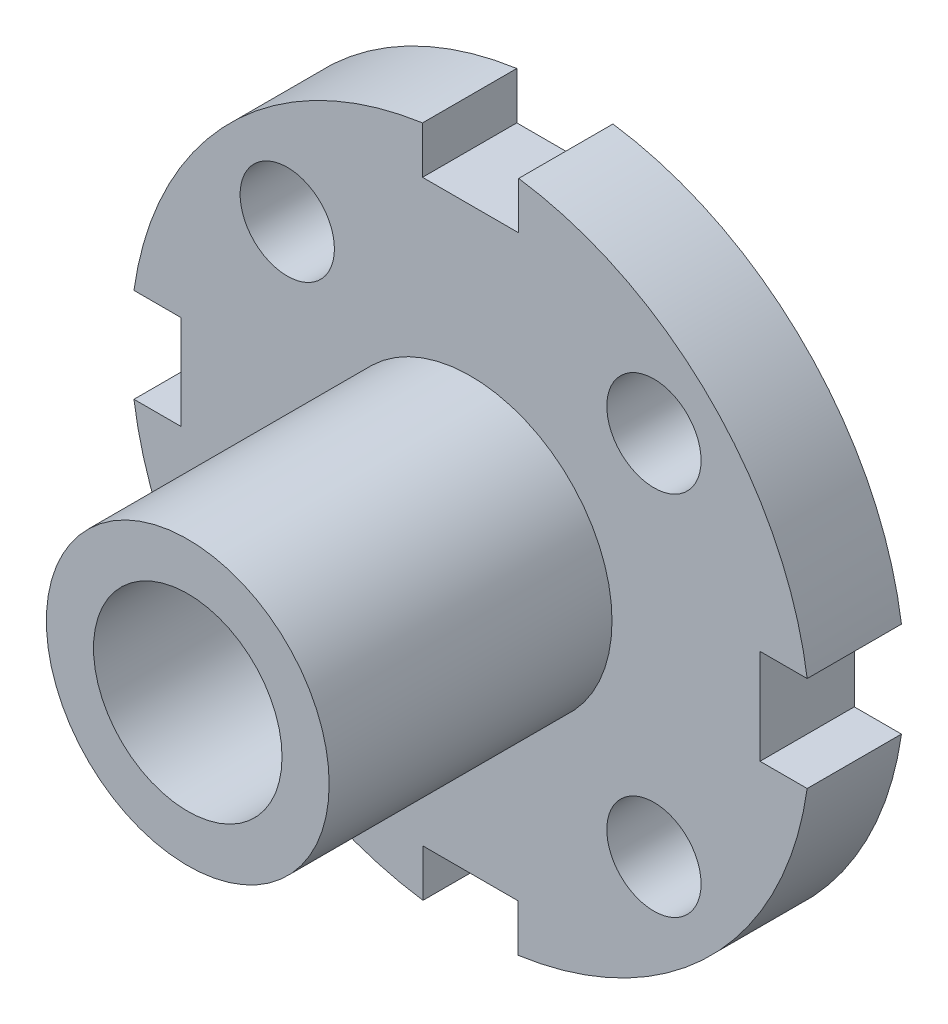
ISO-10303-21;
HEADER;
FILE_DESCRIPTION(('STEP AP214'),'2;1');
FILE_NAME('part.step','',(''),(''),'','','');
FILE_SCHEMA(('AUTOMOTIVE_DESIGN { 1 0 10303 214 1 1 1 1 }'));
ENDSEC;
DATA;
#1=APPLICATION_CONTEXT('core data for automotive mechanical design processes');
#2=APPLICATION_PROTOCOL_DEFINITION('international standard','automotive_design',2000,#1);
#3=PRODUCT_CONTEXT('',#1,'mechanical');
#4=PRODUCT('Part','Part','',(#3));
#5=PRODUCT_RELATED_PRODUCT_CATEGORY('part','',(#4));
#6=PRODUCT_DEFINITION_FORMATION('','',#4);
#7=PRODUCT_DEFINITION_CONTEXT('part definition',#1,'design');
#8=PRODUCT_DEFINITION('design','',#6,#7);
#9=PRODUCT_DEFINITION_SHAPE('','',#8);
#10=(LENGTH_UNIT() NAMED_UNIT(*) SI_UNIT(.MILLI.,.METRE.));
#11=(NAMED_UNIT(*) PLANE_ANGLE_UNIT() SI_UNIT($,.RADIAN.));
#12=(NAMED_UNIT(*) SI_UNIT($,.STERADIAN.) SOLID_ANGLE_UNIT());
#13=UNCERTAINTY_MEASURE_WITH_UNIT(LENGTH_MEASURE(1.E-05),#10,'distance_accuracy_value','');
#14=(GEOMETRIC_REPRESENTATION_CONTEXT(3) GLOBAL_UNCERTAINTY_ASSIGNED_CONTEXT((#13)) GLOBAL_UNIT_ASSIGNED_CONTEXT((#10,
#11,#12)) REPRESENTATION_CONTEXT('',''));
#15=CARTESIAN_POINT('',(0.,0.,0.));
#16=DIRECTION('',(0.,0.,1.));
#17=DIRECTION('',(1.,0.,0.));
#18=AXIS2_PLACEMENT_3D('',#15,#16,#17);
#19=CARTESIAN_POINT('',(-5.09901951359279,30.6931365951495,10.));
#20=DIRECTION('',(-1.,0.,0.));
#21=DIRECTION('',(0.,0.,1.));
#22=AXIS2_PLACEMENT_3D('',#19,#20,#21);
#23=PLANE('',#22);
#24=DIRECTION('',(0.,1.,0.));
#25=VECTOR('',#24,1.);
#26=CARTESIAN_POINT('',(-5.09901951359279,30.6931365951495,0.));
#27=LINE('',#26,#25);
#28=CARTESIAN_POINT('',(-5.09901951359279,30.6931365951495,0.));
#29=VERTEX_POINT('',#28);
#30=CARTESIAN_POINT('',(-5.09901951359279,35.6931365951495,0.));
#31=VERTEX_POINT('',#30);
#32=EDGE_CURVE('E194',#29,#31,#27,.T.);
#33=ORIENTED_EDGE('',*,*,#32,.T.);
#34=DIRECTION('',(0.,0.,-1.));
#35=VECTOR('',#34,1.);
#36=CARTESIAN_POINT('',(-5.09901951359279,35.6931365951495,10.));
#37=LINE('',#36,#35);
#38=CARTESIAN_POINT('',(-5.09901951359279,35.6931365951495,10.));
#39=VERTEX_POINT('',#38);
#40=EDGE_CURVE('E53',#39,#31,#37,.T.);
#41=ORIENTED_EDGE('',*,*,#40,.F.);
#42=DIRECTION('',(0.,1.,0.));
#43=VECTOR('',#42,1.);
#44=CARTESIAN_POINT('',(-5.09901951359279,30.6931365951495,10.));
#45=LINE('',#44,#43);
#46=CARTESIAN_POINT('',(-5.09901951359279,30.6931365951495,10.));
#47=VERTEX_POINT('',#46);
#48=EDGE_CURVE('E128',#47,#39,#45,.T.);
#49=ORIENTED_EDGE('',*,*,#48,.F.);
#50=DIRECTION('',(0.,0.,-1.));
#51=VECTOR('',#50,1.);
#52=CARTESIAN_POINT('',(-5.09901951359279,30.6931365951495,10.));
#53=LINE('',#52,#51);
#54=EDGE_CURVE('E11',#47,#29,#53,.T.);
#55=ORIENTED_EDGE('',*,*,#54,.T.);
#56=EDGE_LOOP('',(#33,#41,#49,#55));
#57=FACE_BOUND('',#56,.T.);
#58=ADVANCED_FACE('F44',(#57),#23,.F.);
#59=CARTESIAN_POINT('',(0.,0.,10.));
#60=DIRECTION('',(0.,0.,-1.));
#61=DIRECTION('',(-1.,0.,0.));
#62=AXIS2_PLACEMENT_3D('',#59,#60,#61);
#63=CYLINDRICAL_SURFACE('',#62,36.0555127546399);
#64=CARTESIAN_POINT('',(0.,0.,0.));
#65=DIRECTION('',(0.,0.,1.));
#66=DIRECTION('',(1.,0.,0.));
#67=AXIS2_PLACEMENT_3D('',#64,#65,#66);
#68=CIRCLE('',#67,36.0555127546399);
#69=CARTESIAN_POINT('',(-35.7071421427143,5.,0.));
#70=VERTEX_POINT('',#69);
#71=EDGE_CURVE('E198',#31,#70,#68,.T.);
#72=ORIENTED_EDGE('',*,*,#71,.T.);
#73=DIRECTION('',(0.,0.,-1.));
#74=VECTOR('',#73,1.);
#75=CARTESIAN_POINT('',(-35.7071421427143,5.,10.));
#76=LINE('',#75,#74);
#77=CARTESIAN_POINT('',(-35.7071421427143,5.,10.));
#78=VERTEX_POINT('',#77);
#79=EDGE_CURVE('E260',#78,#70,#76,.T.);
#80=ORIENTED_EDGE('',*,*,#79,.F.);
#81=CARTESIAN_POINT('',(0.,0.,10.));
#82=DIRECTION('',(0.,0.,1.));
#83=DIRECTION('',(1.,0.,0.));
#84=AXIS2_PLACEMENT_3D('',#81,#82,#83);
#85=CIRCLE('',#84,36.0555127546399);
#86=EDGE_CURVE('E266',#39,#78,#85,.T.);
#87=ORIENTED_EDGE('',*,*,#86,.F.);
#88=ORIENTED_EDGE('',*,*,#40,.T.);
#89=EDGE_LOOP('',(#72,#80,#87,#88));
#90=FACE_BOUND('',#89,.T.);
#91=ADVANCED_FACE('F262',(#90),#63,.T.);
#92=CARTESIAN_POINT('',(-30.7071421427143,5.,10.));
#93=DIRECTION('',(0.,1.,0.));
#94=DIRECTION('',(-1.,0.,0.));
#95=AXIS2_PLACEMENT_3D('',#92,#93,#94);
#96=PLANE('',#95);
#97=DIRECTION('',(1.,0.,0.));
#98=VECTOR('',#97,1.);
#99=CARTESIAN_POINT('',(-30.7071421427143,5.,0.));
#100=LINE('',#99,#98);
#101=CARTESIAN_POINT('',(-30.7071421427143,5.,0.));
#102=VERTEX_POINT('',#101);
#103=EDGE_CURVE('E200',#70,#102,#100,.T.);
#104=ORIENTED_EDGE('',*,*,#103,.T.);
#105=DIRECTION('',(0.,0.,-1.));
#106=VECTOR('',#105,1.);
#107=CARTESIAN_POINT('',(-30.7071421427143,5.,10.));
#108=LINE('',#107,#106);
#109=CARTESIAN_POINT('',(-30.7071421427143,5.,10.));
#110=VERTEX_POINT('',#109);
#111=EDGE_CURVE('E255',#110,#102,#108,.T.);
#112=ORIENTED_EDGE('',*,*,#111,.F.);
#113=DIRECTION('',(1.,0.,0.));
#114=VECTOR('',#113,1.);
#115=CARTESIAN_POINT('',(-30.7071421427143,5.,10.));
#116=LINE('',#115,#114);
#117=EDGE_CURVE('E281',#78,#110,#116,.T.);
#118=ORIENTED_EDGE('',*,*,#117,.F.);
#119=ORIENTED_EDGE('',*,*,#79,.T.);
#120=EDGE_LOOP('',(#104,#112,#118,#119));
#121=FACE_BOUND('',#120,.T.);
#122=ADVANCED_FACE('F274',(#121),#96,.F.);
#123=CARTESIAN_POINT('',(-30.7071421427143,0.,10.));
#124=DIRECTION('',(1.,0.,0.));
#125=DIRECTION('',(0.,0.,-1.));
#126=AXIS2_PLACEMENT_3D('',#123,#124,#125);
#127=PLANE('',#126);
#128=DIRECTION('',(0.,-1.,0.));
#129=VECTOR('',#128,1.);
#130=CARTESIAN_POINT('',(-30.7071421427143,0.,0.));
#131=LINE('',#130,#129);
#132=CARTESIAN_POINT('',(-30.7071421427143,-5.,0.));
#133=VERTEX_POINT('',#132);
#134=EDGE_CURVE('E205',#102,#133,#131,.T.);
#135=ORIENTED_EDGE('',*,*,#134,.T.);
#136=DIRECTION('',(0.,0.,-1.));
#137=VECTOR('',#136,1.);
#138=CARTESIAN_POINT('',(-30.7071421427143,-5.,10.));
#139=LINE('',#138,#137);
#140=CARTESIAN_POINT('',(-30.7071421427143,-5.,10.));
#141=VERTEX_POINT('',#140);
#142=EDGE_CURVE('E253',#141,#133,#139,.T.);
#143=ORIENTED_EDGE('',*,*,#142,.F.);
#144=DIRECTION('',(0.,-1.,0.));
#145=VECTOR('',#144,1.);
#146=CARTESIAN_POINT('',(-30.7071421427143,0.,10.));
#147=LINE('',#146,#145);
#148=EDGE_CURVE('E282',#110,#141,#147,.T.);
#149=ORIENTED_EDGE('',*,*,#148,.F.);
#150=ORIENTED_EDGE('',*,*,#111,.T.);
#151=EDGE_LOOP('',(#135,#143,#149,#150));
#152=FACE_BOUND('',#151,.T.);
#153=ADVANCED_FACE('F276',(#152),#127,.F.);
#154=CARTESIAN_POINT('',(-30.7071421427143,-5.,10.));
#155=DIRECTION('',(0.,-1.,0.));
#156=DIRECTION('',(0.,0.,-1.));
#157=AXIS2_PLACEMENT_3D('',#154,#155,#156);
#158=PLANE('',#157);
#159=DIRECTION('',(-1.,0.,0.));
#160=VECTOR('',#159,1.);
#161=CARTESIAN_POINT('',(-30.7071421427143,-5.,0.));
#162=LINE('',#161,#160);
#163=CARTESIAN_POINT('',(-35.7071421427143,-4.99999999999999,0.));
#164=VERTEX_POINT('',#163);
#165=EDGE_CURVE('E204',#133,#164,#162,.T.);
#166=ORIENTED_EDGE('',*,*,#165,.T.);
#167=DIRECTION('',(0.,0.,-1.));
#168=VECTOR('',#167,1.);
#169=CARTESIAN_POINT('',(-35.7071421427143,-4.99999999999999,10.));
#170=LINE('',#169,#168);
#171=CARTESIAN_POINT('',(-35.7071421427143,-4.99999999999999,10.));
#172=VERTEX_POINT('',#171);
#173=EDGE_CURVE('E246',#172,#164,#170,.T.);
#174=ORIENTED_EDGE('',*,*,#173,.F.);
#175=DIRECTION('',(-1.,0.,0.));
#176=VECTOR('',#175,1.);
#177=CARTESIAN_POINT('',(-30.7071421427143,-5.,10.));
#178=LINE('',#177,#176);
#179=EDGE_CURVE('E285',#141,#172,#178,.T.);
#180=ORIENTED_EDGE('',*,*,#179,.F.);
#181=ORIENTED_EDGE('',*,*,#142,.T.);
#182=EDGE_LOOP('',(#166,#174,#180,#181));
#183=FACE_BOUND('',#182,.T.);
#184=ADVANCED_FACE('F372',(#183),#158,.F.);
#185=CARTESIAN_POINT('',(0.,0.,10.));
#186=DIRECTION('',(0.,0.,-1.));
#187=DIRECTION('',(-1.,0.,0.));
#188=AXIS2_PLACEMENT_3D('',#185,#186,#187);
#189=CYLINDRICAL_SURFACE('',#188,36.0555127546399);
#190=CARTESIAN_POINT('',(0.,0.,0.));
#191=DIRECTION('',(0.,0.,1.));
#192=DIRECTION('',(1.,0.,0.));
#193=AXIS2_PLACEMENT_3D('',#190,#191,#192);
#194=CIRCLE('',#193,36.0555127546399);
#195=CARTESIAN_POINT('',(-5.04878164297401,-35.7002773647708,0.));
#196=VERTEX_POINT('',#195);
#197=EDGE_CURVE('E206',#164,#196,#194,.T.);
#198=ORIENTED_EDGE('',*,*,#197,.T.);
#199=DIRECTION('',(0.,0.,-1.));
#200=VECTOR('',#199,1.);
#201=CARTESIAN_POINT('',(-5.04878164297401,-35.7002773647708,10.));
#202=LINE('',#201,#200);
#203=CARTESIAN_POINT('',(-5.04878164297401,-35.7002773647708,10.));
#204=VERTEX_POINT('',#203);
#205=EDGE_CURVE('E243',#204,#196,#202,.T.);
#206=ORIENTED_EDGE('',*,*,#205,.F.);
#207=CARTESIAN_POINT('',(0.,0.,10.));
#208=DIRECTION('',(0.,0.,1.));
#209=DIRECTION('',(1.,0.,0.));
#210=AXIS2_PLACEMENT_3D('',#207,#208,#209);
#211=CIRCLE('',#210,36.0555127546399);
#212=EDGE_CURVE('E288',#172,#204,#211,.T.);
#213=ORIENTED_EDGE('',*,*,#212,.F.);
#214=ORIENTED_EDGE('',*,*,#173,.T.);
#215=EDGE_LOOP('',(#198,#206,#213,#214));
#216=FACE_BOUND('',#215,.T.);
#217=ADVANCED_FACE('F380',(#216),#189,.T.);
#218=CARTESIAN_POINT('',(-5.04878164297401,-30.7002773647708,10.));
#219=DIRECTION('',(-1.,0.,0.));
#220=DIRECTION('',(0.,-1.,0.));
#221=AXIS2_PLACEMENT_3D('',#218,#219,#220);
#222=PLANE('',#221);
#223=DIRECTION('',(0.,1.,0.));
#224=VECTOR('',#223,1.);
#225=CARTESIAN_POINT('',(-5.04878164297401,-30.7002773647708,0.));
#226=LINE('',#225,#224);
#227=CARTESIAN_POINT('',(-5.04878164297401,-30.7002773647708,0.));
#228=VERTEX_POINT('',#227);
#229=EDGE_CURVE('E208',#196,#228,#226,.T.);
#230=ORIENTED_EDGE('',*,*,#229,.T.);
#231=DIRECTION('',(0.,0.,-1.));
#232=VECTOR('',#231,1.);
#233=CARTESIAN_POINT('',(-5.04878164297401,-30.7002773647708,10.));
#234=LINE('',#233,#232);
#235=CARTESIAN_POINT('',(-5.04878164297401,-30.7002773647708,10.));
#236=VERTEX_POINT('',#235);
#237=EDGE_CURVE('E244',#236,#228,#234,.T.);
#238=ORIENTED_EDGE('',*,*,#237,.F.);
#239=DIRECTION('',(0.,1.,0.));
#240=VECTOR('',#239,1.);
#241=CARTESIAN_POINT('',(-5.04878164297401,-30.7002773647708,10.));
#242=LINE('',#241,#240);
#243=EDGE_CURVE('E295',#204,#236,#242,.T.);
#244=ORIENTED_EDGE('',*,*,#243,.F.);
#245=ORIENTED_EDGE('',*,*,#205,.T.);
#246=EDGE_LOOP('',(#230,#238,#244,#245));
#247=FACE_BOUND('',#246,.T.);
#248=ADVANCED_FACE('F381',(#247),#222,.F.);
#249=CARTESIAN_POINT('',(0.,-30.7002773647708,10.));
#250=DIRECTION('',(0.,1.,0.));
#251=DIRECTION('',(0.,0.,1.));
#252=AXIS2_PLACEMENT_3D('',#249,#250,#251);
#253=PLANE('',#252);
#254=DIRECTION('',(1.,0.,0.));
#255=VECTOR('',#254,1.);
#256=CARTESIAN_POINT('',(0.,-30.7002773647708,0.));
#257=LINE('',#256,#255);
#258=CARTESIAN_POINT('',(5.04878164297401,-30.7002773647708,0.));
#259=VERTEX_POINT('',#258);
#260=EDGE_CURVE('E211',#228,#259,#257,.T.);
#261=ORIENTED_EDGE('',*,*,#260,.T.);
#262=DIRECTION('',(0.,0.,-1.));
#263=VECTOR('',#262,1.);
#264=CARTESIAN_POINT('',(5.04878164297401,-30.7002773647708,10.));
#265=LINE('',#264,#263);
#266=CARTESIAN_POINT('',(5.04878164297401,-30.7002773647708,10.));
#267=VERTEX_POINT('',#266);
#268=EDGE_CURVE('E239',#267,#259,#265,.T.);
#269=ORIENTED_EDGE('',*,*,#268,.F.);
#270=DIRECTION('',(1.,0.,0.));
#271=VECTOR('',#270,1.);
#272=CARTESIAN_POINT('',(0.,-30.7002773647708,10.));
#273=LINE('',#272,#271);
#274=EDGE_CURVE('E294',#236,#267,#273,.T.);
#275=ORIENTED_EDGE('',*,*,#274,.F.);
#276=ORIENTED_EDGE('',*,*,#237,.T.);
#277=EDGE_LOOP('',(#261,#269,#275,#276));
#278=FACE_BOUND('',#277,.T.);
#279=ADVANCED_FACE('F384',(#278),#253,.F.);
#280=CARTESIAN_POINT('',(5.04878164297401,-30.7002773647708,10.));
#281=DIRECTION('',(1.,0.,0.));
#282=DIRECTION('',(0.,1.,0.));
#283=AXIS2_PLACEMENT_3D('',#280,#281,#282);
#284=PLANE('',#283);
#285=DIRECTION('',(0.,-1.,0.));
#286=VECTOR('',#285,1.);
#287=CARTESIAN_POINT('',(5.04878164297401,-30.7002773647708,0.));
#288=LINE('',#287,#286);
#289=CARTESIAN_POINT('',(5.04878164297399,-35.7002773647709,0.));
#290=VERTEX_POINT('',#289);
#291=EDGE_CURVE('E213',#259,#290,#288,.T.);
#292=ORIENTED_EDGE('',*,*,#291,.T.);
#293=DIRECTION('',(0.,0.,-1.));
#294=VECTOR('',#293,1.);
#295=CARTESIAN_POINT('',(5.04878164297399,-35.7002773647709,10.));
#296=LINE('',#295,#294);
#297=CARTESIAN_POINT('',(5.04878164297399,-35.7002773647709,10.));
#298=VERTEX_POINT('',#297);
#299=EDGE_CURVE('E237',#298,#290,#296,.T.);
#300=ORIENTED_EDGE('',*,*,#299,.F.);
#301=DIRECTION('',(0.,-1.,0.));
#302=VECTOR('',#301,1.);
#303=CARTESIAN_POINT('',(5.04878164297401,-30.7002773647708,10.));
#304=LINE('',#303,#302);
#305=EDGE_CURVE('E297',#267,#298,#304,.T.);
#306=ORIENTED_EDGE('',*,*,#305,.F.);
#307=ORIENTED_EDGE('',*,*,#268,.T.);
#308=EDGE_LOOP('',(#292,#300,#306,#307));
#309=FACE_BOUND('',#308,.T.);
#310=ADVANCED_FACE('F386',(#309),#284,.F.);
#311=CARTESIAN_POINT('',(0.,0.,10.));
#312=DIRECTION('',(0.,0.,-1.));
#313=DIRECTION('',(-1.,0.,0.));
#314=AXIS2_PLACEMENT_3D('',#311,#312,#313);
#315=CYLINDRICAL_SURFACE('',#314,36.0555127546399);
#316=CARTESIAN_POINT('',(0.,0.,0.));
#317=DIRECTION('',(0.,0.,1.));
#318=DIRECTION('',(1.,0.,0.));
#319=AXIS2_PLACEMENT_3D('',#316,#317,#318);
#320=CIRCLE('',#319,36.0555127546399);
#321=CARTESIAN_POINT('',(35.7002773647708,-5.04878164297401,0.));
#322=VERTEX_POINT('',#321);
#323=EDGE_CURVE('E214',#290,#322,#320,.T.);
#324=ORIENTED_EDGE('',*,*,#323,.T.);
#325=DIRECTION('',(0.,0.,-1.));
#326=VECTOR('',#325,1.);
#327=CARTESIAN_POINT('',(35.7002773647708,-5.04878164297401,10.));
#328=LINE('',#327,#326);
#329=CARTESIAN_POINT('',(35.7002773647708,-5.04878164297401,10.));
#330=VERTEX_POINT('',#329);
#331=EDGE_CURVE('E231',#330,#322,#328,.T.);
#332=ORIENTED_EDGE('',*,*,#331,.F.);
#333=CARTESIAN_POINT('',(0.,0.,10.));
#334=DIRECTION('',(0.,0.,1.));
#335=DIRECTION('',(1.,0.,0.));
#336=AXIS2_PLACEMENT_3D('',#333,#334,#335);
#337=CIRCLE('',#336,36.0555127546399);
#338=EDGE_CURVE('E300',#298,#330,#337,.T.);
#339=ORIENTED_EDGE('',*,*,#338,.F.);
#340=ORIENTED_EDGE('',*,*,#299,.T.);
#341=EDGE_LOOP('',(#324,#332,#339,#340));
#342=FACE_BOUND('',#341,.T.);
#343=ADVANCED_FACE('F395',(#342),#315,.T.);
#344=CARTESIAN_POINT('',(30.7002773647708,-5.04878164297401,10.));
#345=DIRECTION('',(0.,-1.,0.));
#346=DIRECTION('',(0.,0.,-1.));
#347=AXIS2_PLACEMENT_3D('',#344,#345,#346);
#348=PLANE('',#347);
#349=DIRECTION('',(-1.,0.,0.));
#350=VECTOR('',#349,1.);
#351=CARTESIAN_POINT('',(30.7002773647708,-5.04878164297401,0.));
#352=LINE('',#351,#350);
#353=CARTESIAN_POINT('',(30.7002773647708,-5.04878164297401,0.));
#354=VERTEX_POINT('',#353);
#355=EDGE_CURVE('E220',#322,#354,#352,.T.);
#356=ORIENTED_EDGE('',*,*,#355,.T.);
#357=DIRECTION('',(0.,0.,-1.));
#358=VECTOR('',#357,1.);
#359=CARTESIAN_POINT('',(30.7002773647708,-5.04878164297401,10.));
#360=LINE('',#359,#358);
#361=CARTESIAN_POINT('',(30.7002773647708,-5.04878164297401,10.));
#362=VERTEX_POINT('',#361);
#363=EDGE_CURVE('E228',#362,#354,#360,.T.);
#364=ORIENTED_EDGE('',*,*,#363,.F.);
#365=DIRECTION('',(-1.,0.,0.));
#366=VECTOR('',#365,1.);
#367=CARTESIAN_POINT('',(30.7002773647708,-5.04878164297401,10.));
#368=LINE('',#367,#366);
#369=EDGE_CURVE('E298',#330,#362,#368,.T.);
#370=ORIENTED_EDGE('',*,*,#369,.F.);
#371=ORIENTED_EDGE('',*,*,#331,.T.);
#372=EDGE_LOOP('',(#356,#364,#370,#371));
#373=FACE_BOUND('',#372,.T.);
#374=ADVANCED_FACE('F308',(#373),#348,.F.);
#375=CARTESIAN_POINT('',(30.7002773647708,0.,10.));
#376=DIRECTION('',(-1.,0.,0.));
#377=DIRECTION('',(0.,0.,1.));
#378=AXIS2_PLACEMENT_3D('',#375,#376,#377);
#379=PLANE('',#378);
#380=DIRECTION('',(0.,1.,0.));
#381=VECTOR('',#380,1.);
#382=CARTESIAN_POINT('',(30.7002773647708,0.,0.));
#383=LINE('',#382,#381);
#384=CARTESIAN_POINT('',(30.7002773647708,5.04878164297401,0.));
#385=VERTEX_POINT('',#384);
#386=EDGE_CURVE('E219',#354,#385,#383,.T.);
#387=ORIENTED_EDGE('',*,*,#386,.T.);
#388=DIRECTION('',(0.,0.,-1.));
#389=VECTOR('',#388,1.);
#390=CARTESIAN_POINT('',(30.7002773647708,5.04878164297401,10.));
#391=LINE('',#390,#389);
#392=CARTESIAN_POINT('',(30.7002773647708,5.04878164297401,10.));
#393=VERTEX_POINT('',#392);
#394=EDGE_CURVE('E181',#393,#385,#391,.T.);
#395=ORIENTED_EDGE('',*,*,#394,.F.);
#396=DIRECTION('',(0.,1.,0.));
#397=VECTOR('',#396,1.);
#398=CARTESIAN_POINT('',(30.7002773647708,0.,10.));
#399=LINE('',#398,#397);
#400=EDGE_CURVE('E171',#362,#393,#399,.T.);
#401=ORIENTED_EDGE('',*,*,#400,.F.);
#402=ORIENTED_EDGE('',*,*,#363,.T.);
#403=EDGE_LOOP('',(#387,#395,#401,#402));
#404=FACE_BOUND('',#403,.T.);
#405=ADVANCED_FACE('F310',(#404),#379,.F.);
#406=CARTESIAN_POINT('',(30.7002773647708,5.04878164297401,10.));
#407=DIRECTION('',(0.,1.,0.));
#408=DIRECTION('',(0.,0.,1.));
#409=AXIS2_PLACEMENT_3D('',#406,#407,#408);
#410=PLANE('',#409);
#411=DIRECTION('',(1.,0.,0.));
#412=VECTOR('',#411,1.);
#413=CARTESIAN_POINT('',(30.7002773647708,5.04878164297401,0.));
#414=LINE('',#413,#412);
#415=CARTESIAN_POINT('',(35.7002773647708,5.04878164297401,0.));
#416=VERTEX_POINT('',#415);
#417=EDGE_CURVE('E185',#385,#416,#414,.T.);
#418=ORIENTED_EDGE('',*,*,#417,.T.);
#419=DIRECTION('',(0.,0.,-1.));
#420=VECTOR('',#419,1.);
#421=CARTESIAN_POINT('',(35.7002773647708,5.04878164297401,10.));
#422=LINE('',#421,#420);
#423=CARTESIAN_POINT('',(35.7002773647708,5.04878164297401,10.));
#424=VERTEX_POINT('',#423);
#425=EDGE_CURVE('E179',#424,#416,#422,.T.);
#426=ORIENTED_EDGE('',*,*,#425,.F.);
#427=DIRECTION('',(1.,0.,0.));
#428=VECTOR('',#427,1.);
#429=CARTESIAN_POINT('',(30.7002773647708,5.04878164297401,10.));
#430=LINE('',#429,#428);
#431=EDGE_CURVE('E169',#393,#424,#430,.T.);
#432=ORIENTED_EDGE('',*,*,#431,.F.);
#433=ORIENTED_EDGE('',*,*,#394,.T.);
#434=EDGE_LOOP('',(#418,#426,#432,#433));
#435=FACE_BOUND('',#434,.T.);
#436=ADVANCED_FACE('F177',(#435),#410,.F.);
#437=CARTESIAN_POINT('',(0.,0.,10.));
#438=DIRECTION('',(0.,0.,-1.));
#439=DIRECTION('',(-1.,0.,0.));
#440=AXIS2_PLACEMENT_3D('',#437,#438,#439);
#441=CYLINDRICAL_SURFACE('',#440,36.0555127546399);
#442=CARTESIAN_POINT('',(0.,0.,0.));
#443=DIRECTION('',(0.,0.,1.));
#444=DIRECTION('',(1.,0.,0.));
#445=AXIS2_PLACEMENT_3D('',#442,#443,#444);
#446=CIRCLE('',#445,36.0555127546399);
#447=CARTESIAN_POINT('',(5.09901951359279,35.6931365951495,0.));
#448=VERTEX_POINT('',#447);
#449=EDGE_CURVE('E117',#416,#448,#446,.T.);
#450=ORIENTED_EDGE('',*,*,#449,.T.);
#451=DIRECTION('',(0.,0.,-1.));
#452=VECTOR('',#451,1.);
#453=CARTESIAN_POINT('',(5.09901951359279,35.6931365951495,10.));
#454=LINE('',#453,#452);
#455=CARTESIAN_POINT('',(5.09901951359279,35.6931365951495,10.));
#456=VERTEX_POINT('',#455);
#457=EDGE_CURVE('E184',#456,#448,#454,.T.);
#458=ORIENTED_EDGE('',*,*,#457,.F.);
#459=CARTESIAN_POINT('',(0.,0.,10.));
#460=DIRECTION('',(0.,0.,1.));
#461=DIRECTION('',(1.,0.,0.));
#462=AXIS2_PLACEMENT_3D('',#459,#460,#461);
#463=CIRCLE('',#462,36.0555127546399);
#464=EDGE_CURVE('E174',#424,#456,#463,.T.);
#465=ORIENTED_EDGE('',*,*,#464,.F.);
#466=ORIENTED_EDGE('',*,*,#425,.T.);
#467=EDGE_LOOP('',(#450,#458,#465,#466));
#468=FACE_BOUND('',#467,.T.);
#469=ADVANCED_FACE('F187',(#468),#441,.T.);
#470=CARTESIAN_POINT('',(5.09901951359279,30.6931365951495,10.));
#471=DIRECTION('',(1.,0.,0.));
#472=DIRECTION('',(0.,0.,-1.));
#473=AXIS2_PLACEMENT_3D('',#470,#471,#472);
#474=PLANE('',#473);
#475=DIRECTION('',(0.,-1.,0.));
#476=VECTOR('',#475,1.);
#477=CARTESIAN_POINT('',(5.09901951359279,30.6931365951495,0.));
#478=LINE('',#477,#476);
#479=CARTESIAN_POINT('',(5.09901951359279,30.6931365951495,0.));
#480=VERTEX_POINT('',#479);
#481=EDGE_CURVE('E121',#448,#480,#478,.T.);
#482=ORIENTED_EDGE('',*,*,#481,.T.);
#483=DIRECTION('',(0.,0.,-1.));
#484=VECTOR('',#483,1.);
#485=CARTESIAN_POINT('',(5.09901951359279,30.6931365951495,10.));
#486=LINE('',#485,#484);
#487=CARTESIAN_POINT('',(5.09901951359279,30.6931365951495,10.));
#488=VERTEX_POINT('',#487);
#489=EDGE_CURVE('E188',#488,#480,#486,.T.);
#490=ORIENTED_EDGE('',*,*,#489,.F.);
#491=DIRECTION('',(0.,-1.,0.));
#492=VECTOR('',#491,1.);
#493=CARTESIAN_POINT('',(5.09901951359279,30.6931365951495,10.));
#494=LINE('',#493,#492);
#495=EDGE_CURVE('E190',#456,#488,#494,.T.);
#496=ORIENTED_EDGE('',*,*,#495,.F.);
#497=ORIENTED_EDGE('',*,*,#457,.T.);
#498=EDGE_LOOP('',(#482,#490,#496,#497));
#499=FACE_BOUND('',#498,.T.);
#500=ADVANCED_FACE('F313',(#499),#474,.F.);
#501=CARTESIAN_POINT('',(0.,30.6931365951495,10.));
#502=DIRECTION('',(0.,-1.,0.));
#503=DIRECTION('',(0.,0.,-1.));
#504=AXIS2_PLACEMENT_3D('',#501,#502,#503);
#505=PLANE('',#504);
#506=DIRECTION('',(-1.,0.,0.));
#507=VECTOR('',#506,1.);
#508=CARTESIAN_POINT('',(0.,30.6931365951495,0.));
#509=LINE('',#508,#507);
#510=EDGE_CURVE('E223',#480,#29,#509,.T.);
#511=ORIENTED_EDGE('',*,*,#510,.T.);
#512=ORIENTED_EDGE('',*,*,#54,.F.);
#513=DIRECTION('',(-1.,0.,0.));
#514=VECTOR('',#513,1.);
#515=CARTESIAN_POINT('',(0.,30.6931365951495,10.));
#516=LINE('',#515,#514);
#517=EDGE_CURVE('E64',#488,#47,#516,.T.);
#518=ORIENTED_EDGE('',*,*,#517,.F.);
#519=ORIENTED_EDGE('',*,*,#489,.T.);
#520=EDGE_LOOP('',(#511,#512,#518,#519));
#521=FACE_BOUND('',#520,.T.);
#522=ADVANCED_FACE('F309',(#521),#505,.F.);
#523=CARTESIAN_POINT('',(0.,0.,10.));
#524=DIRECTION('',(0.,0.,1.));
#525=DIRECTION('',(1.,0.,0.));
#526=AXIS2_PLACEMENT_3D('',#523,#524,#525);
#527=PLANE('',#526);
#528=CARTESIAN_POINT('',(0.,0.,10.));
#529=DIRECTION('',(0.,0.,1.));
#530=DIRECTION('',(1.,0.,0.));
#531=AXIS2_PLACEMENT_3D('',#528,#529,#530);
#532=CIRCLE('',#531,15.);
#533=CARTESIAN_POINT('',(15.,0.,10.));
#534=VERTEX_POINT('',#533);
#535=EDGE_CURVE('E336',#534,#534,#532,.T.);
#536=ORIENTED_EDGE('',*,*,#535,.F.);
#537=EDGE_LOOP('',(#536));
#538=FACE_BOUND('',#537,.T.);
#539=CARTESIAN_POINT('',(-19.44543648263,19.4454364826301,10.));
#540=DIRECTION('',(0.,0.,1.));
#541=DIRECTION('',(1.,0.,0.));
#542=AXIS2_PLACEMENT_3D('',#539,#540,#541);
#543=CIRCLE('',#542,5.);
#544=CARTESIAN_POINT('',(-14.44543648263,19.4454364826301,10.));
#545=VERTEX_POINT('',#544);
#546=EDGE_CURVE('E321',#545,#545,#543,.T.);
#547=ORIENTED_EDGE('',*,*,#546,.F.);
#548=EDGE_LOOP('',(#547));
#549=FACE_BOUND('',#548,.T.);
#550=CARTESIAN_POINT('',(-19.44543648263,-19.4454364826301,10.));
#551=DIRECTION('',(0.,0.,1.));
#552=DIRECTION('',(1.,0.,0.));
#553=AXIS2_PLACEMENT_3D('',#550,#551,#552);
#554=CIRCLE('',#553,5.);
#555=CARTESIAN_POINT('',(-14.44543648263,-19.4454364826301,10.));
#556=VERTEX_POINT('',#555);
#557=EDGE_CURVE('E327',#556,#556,#554,.T.);
#558=ORIENTED_EDGE('',*,*,#557,.F.);
#559=EDGE_LOOP('',(#558));
#560=FACE_BOUND('',#559,.T.);
#561=CARTESIAN_POINT('',(19.4454364826301,-19.44543648263,10.));
#562=DIRECTION('',(0.,0.,1.));
#563=DIRECTION('',(1.,0.,0.));
#564=AXIS2_PLACEMENT_3D('',#561,#562,#563);
#565=CIRCLE('',#564,5.);
#566=CARTESIAN_POINT('',(24.4454364826301,-19.44543648263,10.));
#567=VERTEX_POINT('',#566);
#568=EDGE_CURVE('E331',#567,#567,#565,.T.);
#569=ORIENTED_EDGE('',*,*,#568,.F.);
#570=EDGE_LOOP('',(#569));
#571=FACE_BOUND('',#570,.T.);
#572=CARTESIAN_POINT('',(19.44543648263,19.4454364826301,10.));
#573=DIRECTION('',(0.,0.,1.));
#574=DIRECTION('',(1.,0.,0.));
#575=AXIS2_PLACEMENT_3D('',#572,#573,#574);
#576=CIRCLE('',#575,5.00000000000001);
#577=CARTESIAN_POINT('',(24.44543648263,19.4454364826301,10.));
#578=VERTEX_POINT('',#577);
#579=EDGE_CURVE('E312',#578,#578,#576,.T.);
#580=ORIENTED_EDGE('',*,*,#579,.F.);
#581=EDGE_LOOP('',(#580));
#582=FACE_BOUND('',#581,.T.);
#583=ORIENTED_EDGE('',*,*,#517,.T.);
#584=ORIENTED_EDGE('',*,*,#48,.T.);
#585=ORIENTED_EDGE('',*,*,#86,.T.);
#586=ORIENTED_EDGE('',*,*,#117,.T.);
#587=ORIENTED_EDGE('',*,*,#148,.T.);
#588=ORIENTED_EDGE('',*,*,#179,.T.);
#589=ORIENTED_EDGE('',*,*,#212,.T.);
#590=ORIENTED_EDGE('',*,*,#243,.T.);
#591=ORIENTED_EDGE('',*,*,#274,.T.);
#592=ORIENTED_EDGE('',*,*,#305,.T.);
#593=ORIENTED_EDGE('',*,*,#338,.T.);
#594=ORIENTED_EDGE('',*,*,#369,.T.);
#595=ORIENTED_EDGE('',*,*,#400,.T.);
#596=ORIENTED_EDGE('',*,*,#431,.T.);
#597=ORIENTED_EDGE('',*,*,#464,.T.);
#598=ORIENTED_EDGE('',*,*,#495,.T.);
#599=EDGE_LOOP('',(#583,#584,#585,#586,#587,#588,#589,#590,#591,#592,#593,#594,#595,#596,#597,#598));
#600=FACE_BOUND('',#599,.T.);
#601=ADVANCED_FACE('F168',(#538,#549,#560,#571,#582,#600),#527,.T.);
#602=CARTESIAN_POINT('',(0.,0.,0.));
#603=DIRECTION('',(0.,0.,1.));
#604=DIRECTION('',(1.,0.,0.));
#605=AXIS2_PLACEMENT_3D('',#602,#603,#604);
#606=PLANE('',#605);
#607=CARTESIAN_POINT('',(0.,0.,0.));
#608=DIRECTION('',(0.,0.,1.));
#609=DIRECTION('',(1.,0.,0.));
#610=AXIS2_PLACEMENT_3D('',#607,#608,#609);
#611=CIRCLE('',#610,10.);
#612=CARTESIAN_POINT('',(10.,0.,0.));
#613=VERTEX_POINT('',#612);
#614=EDGE_CURVE('E48',#613,#613,#611,.T.);
#615=ORIENTED_EDGE('',*,*,#614,.T.);
#616=EDGE_LOOP('',(#615));
#617=FACE_BOUND('',#616,.T.);
#618=CARTESIAN_POINT('',(-19.44543648263,19.4454364826301,0.));
#619=DIRECTION('',(0.,0.,1.));
#620=DIRECTION('',(1.,0.,0.));
#621=AXIS2_PLACEMENT_3D('',#618,#619,#620);
#622=CIRCLE('',#621,5.);
#623=CARTESIAN_POINT('',(-14.44543648263,19.4454364826301,0.));
#624=VERTEX_POINT('',#623);
#625=EDGE_CURVE('E322',#624,#624,#622,.T.);
#626=ORIENTED_EDGE('',*,*,#625,.T.);
#627=EDGE_LOOP('',(#626));
#628=FACE_BOUND('',#627,.T.);
#629=CARTESIAN_POINT('',(-19.44543648263,-19.4454364826301,0.));
#630=DIRECTION('',(0.,0.,1.));
#631=DIRECTION('',(1.,0.,0.));
#632=AXIS2_PLACEMENT_3D('',#629,#630,#631);
#633=CIRCLE('',#632,5.);
#634=CARTESIAN_POINT('',(-14.44543648263,-19.4454364826301,0.));
#635=VERTEX_POINT('',#634);
#636=EDGE_CURVE('E332',#635,#635,#633,.T.);
#637=ORIENTED_EDGE('',*,*,#636,.T.);
#638=EDGE_LOOP('',(#637));
#639=FACE_BOUND('',#638,.T.);
#640=CARTESIAN_POINT('',(19.4454364826301,-19.44543648263,0.));
#641=DIRECTION('',(0.,0.,1.));
#642=DIRECTION('',(1.,0.,0.));
#643=AXIS2_PLACEMENT_3D('',#640,#641,#642);
#644=CIRCLE('',#643,5.);
#645=CARTESIAN_POINT('',(24.4454364826301,-19.44543648263,0.));
#646=VERTEX_POINT('',#645);
#647=EDGE_CURVE('E318',#646,#646,#644,.T.);
#648=ORIENTED_EDGE('',*,*,#647,.T.);
#649=EDGE_LOOP('',(#648));
#650=FACE_BOUND('',#649,.T.);
#651=CARTESIAN_POINT('',(19.44543648263,19.4454364826301,0.));
#652=DIRECTION('',(0.,0.,1.));
#653=DIRECTION('',(1.,0.,0.));
#654=AXIS2_PLACEMENT_3D('',#651,#652,#653);
#655=CIRCLE('',#654,5.00000000000001);
#656=CARTESIAN_POINT('',(24.44543648263,19.4454364826301,0.));
#657=VERTEX_POINT('',#656);
#658=EDGE_CURVE('E197',#657,#657,#655,.T.);
#659=ORIENTED_EDGE('',*,*,#658,.T.);
#660=EDGE_LOOP('',(#659));
#661=FACE_BOUND('',#660,.T.);
#662=ORIENTED_EDGE('',*,*,#32,.F.);
#663=ORIENTED_EDGE('',*,*,#510,.F.);
#664=ORIENTED_EDGE('',*,*,#481,.F.);
#665=ORIENTED_EDGE('',*,*,#449,.F.);
#666=ORIENTED_EDGE('',*,*,#417,.F.);
#667=ORIENTED_EDGE('',*,*,#386,.F.);
#668=ORIENTED_EDGE('',*,*,#355,.F.);
#669=ORIENTED_EDGE('',*,*,#323,.F.);
#670=ORIENTED_EDGE('',*,*,#291,.F.);
#671=ORIENTED_EDGE('',*,*,#260,.F.);
#672=ORIENTED_EDGE('',*,*,#229,.F.);
#673=ORIENTED_EDGE('',*,*,#197,.F.);
#674=ORIENTED_EDGE('',*,*,#165,.F.);
#675=ORIENTED_EDGE('',*,*,#134,.F.);
#676=ORIENTED_EDGE('',*,*,#103,.F.);
#677=ORIENTED_EDGE('',*,*,#71,.F.);
#678=EDGE_LOOP('',(#662,#663,#664,#665,#666,#667,#668,#669,#670,#671,#672,#673,#674,#675,#676,#677));
#679=FACE_BOUND('',#678,.T.);
#680=ADVANCED_FACE('F269',(#617,#628,#639,#650,#661,#679),#606,.F.);
#681=CARTESIAN_POINT('',(19.44543648263,19.4454364826301,0.));
#682=DIRECTION('',(0.,0.,1.));
#683=DIRECTION('',(1.,0.,0.));
#684=AXIS2_PLACEMENT_3D('',#681,#682,#683);
#685=CYLINDRICAL_SURFACE('',#684,5.00000000000001);
#686=ORIENTED_EDGE('',*,*,#658,.F.);
#687=EDGE_LOOP('',(#686));
#688=FACE_BOUND('',#687,.T.);
#689=ORIENTED_EDGE('',*,*,#579,.T.);
#690=EDGE_LOOP('',(#689));
#691=FACE_BOUND('',#690,.T.);
#692=ADVANCED_FACE('F415',(#688,#691),#685,.F.);
#693=CARTESIAN_POINT('',(19.4454364826301,-19.44543648263,0.));
#694=DIRECTION('',(0.,0.,1.));
#695=DIRECTION('',(1.,0.,0.));
#696=AXIS2_PLACEMENT_3D('',#693,#694,#695);
#697=CYLINDRICAL_SURFACE('',#696,5.);
#698=ORIENTED_EDGE('',*,*,#647,.F.);
#699=EDGE_LOOP('',(#698));
#700=FACE_BOUND('',#699,.T.);
#701=ORIENTED_EDGE('',*,*,#568,.T.);
#702=EDGE_LOOP('',(#701));
#703=FACE_BOUND('',#702,.T.);
#704=ADVANCED_FACE('F416',(#700,#703),#697,.F.);
#705=CARTESIAN_POINT('',(-19.44543648263,-19.4454364826301,0.));
#706=DIRECTION('',(0.,0.,1.));
#707=DIRECTION('',(1.,0.,0.));
#708=AXIS2_PLACEMENT_3D('',#705,#706,#707);
#709=CYLINDRICAL_SURFACE('',#708,5.);
#710=ORIENTED_EDGE('',*,*,#636,.F.);
#711=EDGE_LOOP('',(#710));
#712=FACE_BOUND('',#711,.T.);
#713=ORIENTED_EDGE('',*,*,#557,.T.);
#714=EDGE_LOOP('',(#713));
#715=FACE_BOUND('',#714,.T.);
#716=ADVANCED_FACE('F421',(#712,#715),#709,.F.);
#717=CARTESIAN_POINT('',(-19.44543648263,19.4454364826301,0.));
#718=DIRECTION('',(0.,0.,1.));
#719=DIRECTION('',(1.,0.,0.));
#720=AXIS2_PLACEMENT_3D('',#717,#718,#719);
#721=CYLINDRICAL_SURFACE('',#720,5.);
#722=ORIENTED_EDGE('',*,*,#625,.F.);
#723=EDGE_LOOP('',(#722));
#724=FACE_BOUND('',#723,.T.);
#725=ORIENTED_EDGE('',*,*,#546,.T.);
#726=EDGE_LOOP('',(#725));
#727=FACE_BOUND('',#726,.T.);
#728=ADVANCED_FACE('F419',(#724,#727),#721,.F.);
#729=CARTESIAN_POINT('',(0.,0.,40.));
#730=DIRECTION('',(0.,0.,-1.));
#731=DIRECTION('',(-1.,0.,0.));
#732=AXIS2_PLACEMENT_3D('',#729,#730,#731);
#733=CYLINDRICAL_SURFACE('',#732,15.);
#734=CARTESIAN_POINT('',(0.,0.,40.));
#735=DIRECTION('',(0.,0.,1.));
#736=DIRECTION('',(1.,0.,0.));
#737=AXIS2_PLACEMENT_3D('',#734,#735,#736);
#738=CIRCLE('',#737,15.);
#739=CARTESIAN_POINT('',(15.,0.,40.));
#740=VERTEX_POINT('',#739);
#741=EDGE_CURVE('E324',#740,#740,#738,.T.);
#742=ORIENTED_EDGE('',*,*,#741,.F.);
#743=EDGE_LOOP('',(#742));
#744=FACE_BOUND('',#743,.T.);
#745=ORIENTED_EDGE('',*,*,#535,.T.);
#746=EDGE_LOOP('',(#745));
#747=FACE_BOUND('',#746,.T.);
#748=ADVANCED_FACE('F357',(#744,#747),#733,.T.);
#749=CARTESIAN_POINT('',(0.,0.,40.));
#750=DIRECTION('',(0.,0.,1.));
#751=DIRECTION('',(1.,0.,0.));
#752=AXIS2_PLACEMENT_3D('',#749,#750,#751);
#753=PLANE('',#752);
#754=CARTESIAN_POINT('',(0.,0.,40.));
#755=DIRECTION('',(0.,0.,1.));
#756=DIRECTION('',(1.,0.,0.));
#757=AXIS2_PLACEMENT_3D('',#754,#755,#756);
#758=CIRCLE('',#757,10.);
#759=CARTESIAN_POINT('',(10.,0.,40.));
#760=VERTEX_POINT('',#759);
#761=EDGE_CURVE('E345',#760,#760,#758,.T.);
#762=ORIENTED_EDGE('',*,*,#761,.F.);
#763=EDGE_LOOP('',(#762));
#764=FACE_BOUND('',#763,.T.);
#765=ORIENTED_EDGE('',*,*,#741,.T.);
#766=EDGE_LOOP('',(#765));
#767=FACE_BOUND('',#766,.T.);
#768=ADVANCED_FACE('F353',(#764,#767),#753,.T.);
#769=CARTESIAN_POINT('',(0.,0.,10.));
#770=DIRECTION('',(0.,0.,1.));
#771=DIRECTION('',(1.,0.,0.));
#772=AXIS2_PLACEMENT_3D('',#769,#770,#771);
#773=CYLINDRICAL_SURFACE('',#772,10.);
#774=ORIENTED_EDGE('',*,*,#761,.T.);
#775=EDGE_LOOP('',(#774));
#776=FACE_BOUND('',#775,.T.);
#777=ORIENTED_EDGE('',*,*,#614,.F.);
#778=EDGE_LOOP('',(#777));
#779=FACE_BOUND('',#778,.T.);
#780=ADVANCED_FACE('F355',(#776,#779),#773,.F.);
#781=CLOSED_SHELL('',(#58,#91,#122,#153,#184,#217,#248,#279,#310,#343,#374,#405,#436,#469,#500,
#522,#601,#680,#692,#704,#716,#728,#748,#768,#780));
#782=MANIFOLD_SOLID_BREP('B2',#781);
#783=ADVANCED_BREP_SHAPE_REPRESENTATION('',(#18,#782),#14);
#784=SHAPE_DEFINITION_REPRESENTATION(#9,#783);
ENDSEC;
END-ISO-10303-21;
